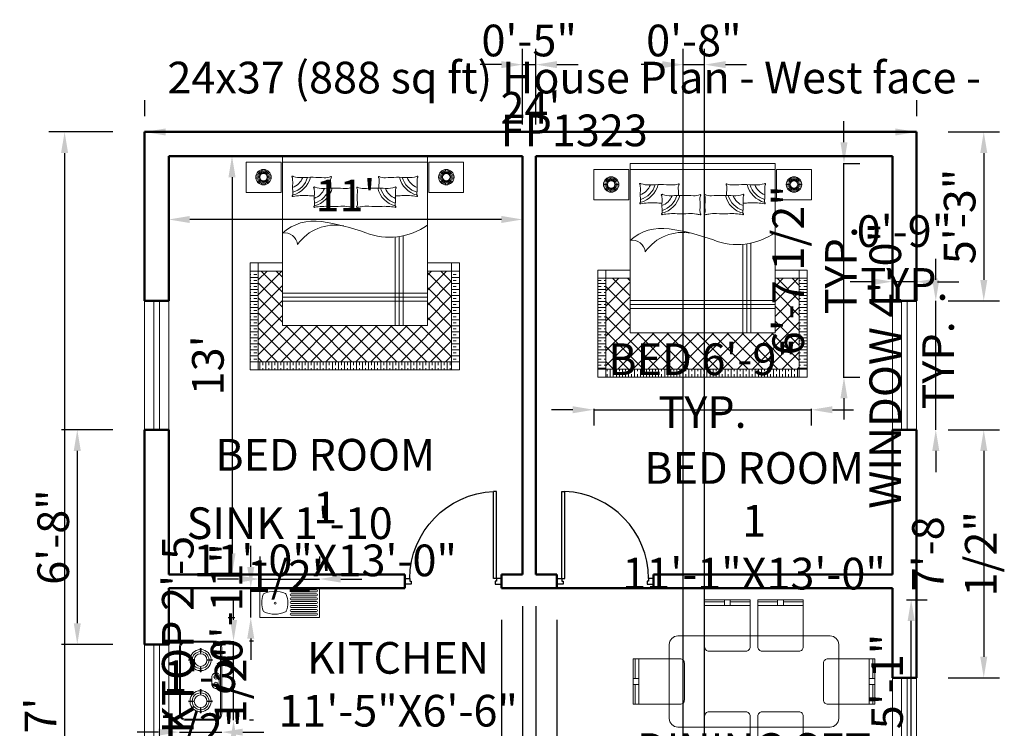
# Model space of a CAD drawing. Units: inches. Extents: x 314 to 688, y 344 to 882.
# Tile 3 of 3: x 321 to 688, y 618 to 882. Entities that reach past the tile are written whole.
import ezdxf

# ---------------------------------------------------------------- set-up
doc = ezdxf.new("R2010")
doc.units = ezdxf.units.IN
doc.header["$MEASUREMENT"] = 0
for name, color, linetype, lineweight in [('A-ANNO-TEXT', 7, 'Continuous', 25), ('A-AREA-IDEN', 7, 'Continuous', 25), ('A-DOOR', 4, 'Continuous', 25), ('A-EQPM', 8, 'Continuous', 18), ('A-FLOR-FIXT', 9, 'Continuous', 18), ('A-FURN', 8, 'Continuous', 18), ('WALL', 7, 'Continuous', 50), ('WINDOW', 2, 'Continuous', 18), ('YQ_DIM', 3, 'Continuous', 18)]:
    doc.layers.add(name, color=color, linetype=linetype, lineweight=lineweight)
doc.styles.add('YQ_DIM', font='SUPEROS.SHX', dxfattribs={"width": 0.8, "bigfont": 'HZDX.SHX'})
doc.dimstyles.new('yqi3_937', dxfattribs={"dimscale": 3.937008, "dimtxt": 3, "dimasz": 2, "dimexe": 1.5, "dimexo": 3, "dimgap": 0.5, "dimtad": 1, "dimdsep": 46, "dimlunit": 4, "dimtxsty": 'YQ_DIM', "dimcen": 0, "dimclrd": 256, "dimclre": 256, "dimclrt": 7, "dimadec": 1, "dimazin": 2, "dimtfac": 1, "dimtix": 1, "dimtmove": 2, "dimatfit": 2, "dimfxl": 1, "dimtolj": 1, "dimtzin": 0, "dimarcsym": 0})

# ---------------------------------------------------------------- blocks, each defined once
blk = doc.blocks.new('*D2')
at = {"layer": 'Defpoints', "color": 0, "transparency": 16777216}
for p in [(367.29, 840.23), (337.46, 396.23), (367.29, 396.23)]:
    blk.add_point(p, dxfattribs=at)
at = {"layer": 'YQ_DIM', "color": 0, "lineweight": -2, "transparency": 16777216}
for p, q in [((355.48, 840.23), (331.55, 840.23)), ((337.46, 832.36), (337.46, 404.11)), ((355.48, 396.23), (331.55, 396.23))]:
    blk.add_line(p, q, dxfattribs=at)
at = {"layer": 'YQ_DIM', "color": 0, "transparency": 16777216}
for points in [[(336.14, 832.36), (338.77, 832.36), (337.46, 840.23)], [(336.14, 404.11), (338.77, 404.11), (337.46, 396.23)]]:
    blk.add_solid(points, dxfattribs=at)
at = {"layer": 'YQ_DIM', "color": 0, "transparency": 16777216, "insert": (328.46, 618.23), "char_height": 11.811, "attachment_point": 5, "rotation": 90, "style": 'YQ_DIM'}
blk.add_mtext("\\A1;37'", dxfattribs=at)
blk = doc.blocks.new('*D3')
at = {"layer": 'Defpoints', "color": 0, "transparency": 16777216}
for p in [(376.29, 831.23), (508.29, 831.23), (376.29, 807.61)]:
    blk.add_point(p, dxfattribs=at)
at = {"layer": 'YQ_DIM', "color": 0, "lineweight": -2, "transparency": 16777216}
for p, q in [((376.29, 819.42), (376.29, 801.71)), ((508.29, 819.42), (508.29, 801.71)), ((500.42, 807.61), (384.17, 807.61))]:
    blk.add_line(p, q, dxfattribs=at)
at = {"layer": 'YQ_DIM', "color": 0, "transparency": 16777216}
for points in [[(384.17, 808.92), (384.17, 806.3), (376.29, 807.61)], [(500.42, 808.92), (500.42, 806.3), (508.29, 807.61)]]:
    blk.add_solid(points, dxfattribs=at)
at = {"layer": 'YQ_DIM', "color": 0, "transparency": 16777216, "insert": (442.29, 816.61), "char_height": 11.811, "attachment_point": 5, "style": 'YQ_DIM'}
blk.add_mtext("\\A1;11'", dxfattribs=at)
blk = doc.blocks.new('*D4')
at = {"layer": 'Defpoints', "color": 0, "transparency": 16777216}
for p in [(376.29, 831.23), (376.29, 675.23), (399.92, 675.23)]:
    blk.add_point(p, dxfattribs=at)
at = {"layer": 'YQ_DIM', "color": 0, "lineweight": -2, "transparency": 16777216}
for p, q in [((388.1, 831.23), (405.82, 831.23)), ((399.92, 823.36), (399.92, 683.11)), ((388.1, 675.23), (405.82, 675.23))]:
    blk.add_line(p, q, dxfattribs=at)
at = {"layer": 'YQ_DIM', "color": 0, "transparency": 16777216}
for points in [[(398.6, 823.36), (401.23, 823.36), (399.92, 831.23)], [(398.6, 683.11), (401.23, 683.11), (399.92, 675.23)]]:
    blk.add_solid(points, dxfattribs=at)
at = {"layer": 'YQ_DIM', "color": 0, "transparency": 16777216, "insert": (390.92, 753.23), "char_height": 11.811, "attachment_point": 5, "rotation": 90, "style": 'YQ_DIM'}
blk.add_mtext("\\A1;13'", dxfattribs=at)
blk = doc.blocks.new('DR_D01')
for p, q in [((-0.45, 0.93), (-0.42, 0.93)), ((-0.45, 0.03), (-0.45, 0.93)), ((-0.42, 0.03), (-0.42, 0.93)), ((-0.5, 0.03), (-0.42, 0.03)), ((-0.5, 0.03), (-0.5, -0.03)), ((-0.45, 0.03), (-0.45, 0)), ((-0.45, 0), (-0.435, 0)), ((-0.435, 0), (-0.435, -0.03)), ((0.435, 0), (0.435, -0.03)), ((0.45, 0), (0.435, 0)), ((0.45, 0.03), (0.45, 0)), ((0.5, 0.03), (0.45, 0.03)), ((0.5, -0.03), (0.5, 0.03)), ((-0.435, -0.03), (-0.5, -0.03)), ((0.435, -0.03), (0.5, -0.03))]:
    blk.add_line(p, q)
blk.add_arc((-0.46, 0.021), 0.91, 0.5915, 87.4664)
blk = doc.blocks.new('WD_WIN4')
for p, q in [((-0.5, 0.5), (0.5, 0.5)), ((-0.5, 0.12), (0.5, 0.12)), ((-0.5, -0.12), (0.5, -0.12)), ((-0.5, -0.5), (0.5, -0.5))]:
    blk.add_line(p, q)
blk = doc.blocks.new('*D8')
at = {"layer": 'Defpoints', "color": 0, "transparency": 16777216}
for p in [(367.29, 840.23), (655.29, 840.23), (655.29, 840.23)]:
    blk.add_point(p, dxfattribs=at)
at = {"layer": 'YQ_DIM', "color": 0, "lineweight": -2, "transparency": 16777216}
for p, q in [((367.29, 852.04), (367.29, 846.14)), ((655.29, 852.04), (655.29, 846.14)), ((375.17, 840.23), (647.42, 840.23))]:
    blk.add_line(p, q, dxfattribs=at)
at = {"layer": 'YQ_DIM', "color": 0, "transparency": 16777216}
for points in [[(375.17, 841.54), (375.17, 838.92), (367.29, 840.23)], [(647.42, 841.54), (647.42, 838.92), (655.29, 840.23)]]:
    blk.add_solid(points, dxfattribs=at)
at = {"layer": 'YQ_DIM', "color": 0, "transparency": 16777216, "insert": (511.29, 849.23), "char_height": 11.811, "attachment_point": 5, "style": 'YQ_DIM'}
blk.add_mtext("\\A1;24'", dxfattribs=at)
blk = doc.blocks.new('BED')
h = blk.add_hatch()
h.set_pattern_fill('TRANS', color=256, scale=12, style=0)
h.set_pattern_definition([(360, (4433.967, -9715.0492), (1e-15, 3), []), (360, (4433.967, -9713.5492), (1e-15, 3), [1.5, -1.5])])
h.paths.add_polyline_path([(48, -103), (52, -103), (52, -58), (48, -58)])
h.paths.add_polyline_path([(-48, -58), (-52, -58), (-52, -103), (-48, -103)])
h = blk.add_hatch()
h.set_pattern_fill('ANSI37', color=256, scale=42, angle=-90, style=0)
h.set_pattern_definition([(315, (7787.1367, 4477.8466), (3.7123106, 3.7123106), []), (45, (7787.1367, 4477.8466), (-3.7123106, 3.7123106), [])])
h.paths.add_polyline_path([(-36, -85), (-36, -58), (-48, -58), (-48, -103), (48, -103), (48, -58), (36, -58), (36, -85)])
h = blk.add_hatch()
h.set_pattern_fill('TRANS', color=256, scale=12, angle=-90, style=0)
h.set_pattern_definition([(270, (4433.967, -9715.0492), (3, -1e-15), []), (270, (4435.467, -9715.0492), (3, -1e-15), [1.5, -1.5])])
h.paths.add_polyline_path([(48, -107), (48, -103), (-48, -103), (-48, -107)])
for p, q in [((-54, -4), (-54, -19)), ((-36.64, -4), (-54, -4)), ((-36.64, -4), (-36.64, -19)), ((-36, -1), (36, -1)), ((-36, -85), (-36, -1)), ((-36, -4), (36, -4)), ((36, -1), (36, -85)), ((36.64, -4), (36.64, -19)), ((36.64, -4), (54, -4)), ((54, -4), (54, -19)), ((-46.88, -10.37), (-48.5, -9.2)), ((-46.62, -10.08), (-47.96, -8.6)), ((-46.31, -9.86), (-47.31, -8.13)), ((-45.96, -9.7), (-46.58, -7.8)), ((-45.58, -9.62), (-45.8, -7.63)), ((-45.2, -9.62), (-45, -7.63)), ((-44.82, -9.7), (-44.21, -7.79)), ((-44.47, -9.85), (-43.48, -8.12)), ((-44.16, -10.08), (-42.83, -8.59)), ((-43.9, -10.36), (-42.29, -9.18)), ((43.9, -10.36), (42.29, -9.18)), ((44.16, -10.08), (42.83, -8.59)), ((44.47, -9.85), (43.48, -8.12)), ((44.82, -9.7), (44.21, -7.79)), ((45.2, -9.62), (45, -7.63)), ((45.58, -9.62), (45.8, -7.63)), ((45.96, -9.7), (46.58, -7.8)), ((46.31, -9.86), (47.31, -8.13)), ((46.62, -10.08), (47.96, -8.6)), ((46.88, -10.37), (48.5, -9.2)), ((-47.23, -11.45), (-49.23, -11.45)), ((-47.19, -11.07), (-49.14, -10.66)), ((-47.19, -11.83), (-49.14, -12.25)), ((-47.07, -10.7), (-48.9, -9.89)), ((-47.07, -12.2), (-48.89, -13.01)), ((-46.87, -12.53), (-48.49, -13.71)), ((-46.62, -12.81), (-47.95, -14.3)), ((-46.3, -13.04), (-47.3, -14.77)), ((-45.95, -13.2), (-46.57, -15.1)), ((-45.58, -13.27), (-45.78, -15.26)), ((-45.19, -13.27), (-44.98, -15.26)), ((-44.82, -13.19), (-44.2, -15.09)), ((-44.47, -13.04), (-43.46, -14.77)), ((-44.16, -12.81), (-42.82, -14.29)), ((-43.9, -12.52), (-42.28, -13.7)), ((-43.71, -10.7), (-41.89, -9.88)), ((-43.71, -12.19), (-41.88, -13)), ((-43.59, -11.06), (-41.64, -10.64)), ((-43.59, -11.83), (-41.63, -12.24)), ((-43.55, -11.44), (-41.55, -11.44)), ((43.55, -11.44), (41.55, -11.44)), ((43.59, -11.83), (41.63, -12.24)), ((43.59, -11.06), (41.64, -10.64)), ((43.71, -12.19), (41.88, -13)), ((43.71, -10.7), (41.89, -9.88)), ((43.9, -12.52), (42.28, -13.7)), ((44.16, -12.81), (42.82, -14.29)), ((44.47, -13.04), (43.46, -14.77)), ((44.82, -13.19), (44.2, -15.09)), ((45.19, -13.27), (44.98, -15.26)), ((45.58, -13.27), (45.78, -15.26)), ((45.95, -13.2), (46.57, -15.1)), ((46.3, -13.04), (47.3, -14.77)), ((46.62, -12.81), (47.95, -14.3)), ((46.87, -12.53), (48.49, -13.71)), ((47.07, -10.7), (48.9, -9.89)), ((47.07, -12.2), (48.89, -13.01)), ((47.19, -11.07), (49.14, -10.66)), ((47.19, -11.83), (49.14, -12.25)), ((47.23, -11.45), (49.23, -11.45)), ((-36.64, -19), (-54, -19)), ((36.64, -19), (54, -19)), ((20, -85), (20, -41.14)), ((22, -85), (22, -40.91)), ((24, -85), (24, -40.55)), ((-52, -54), (-52, -107)), ((-52, -54), (-36, -54)), ((-52, -58), (-36, -58)), ((-48, -54), (-48, -107)), ((36, -54), (52, -54)), ((36, -58), (52, -58)), ((48, -54), (48, -107)), ((52, -54), (52, -107)), ((36, -69), (-36, -69)), ((36, -71), (-36, -71)), ((36, -73), (-36, -73)), ((36, -85), (-36, -85)), ((-52, -103), (52, -103)), ((-52, -107), (52, -107))]:
    blk.add_line(p, q)
for centre, radius in [((-45.39, -11.45), 3.84), ((-45.39, -11.45), 1.84), ((45.39, -11.45), 3.84), ((45.39, -11.45), 1.84)]:
    blk.add_circle(centre, radius)
for centre, radius, start, end in [((-30.92, -11.24), 0.328, 35.8976, 208.6272), ((-42.38, -17.5), 12.73, 27.1629, 28.6272), ((-44.37, -13.89), 13.5, 357.4804, 9.3956), ((10.15, -16.29), 41.07, 177.4804, 184.5075), ((-33.8, -8.61), 8.46, 289.8695, 338.9843), ((-33.8, -8.61), 12.06, 283.8498, 346.0842), ((-33.8, -8.61), 10.71, 286.0319, 344.1205), ((-26.84, 0.13), 11.82, 251.1782, 273.3982), ((-20.92, -99.64), 88.13, 86.2964, 93.3982), ((-14.79, -4.98), 6.73, 266.2964, 294.303), ((-8.24, -13.16), 3.86, 159.0146, 186.273), ((-36.64, -16.28), 24.71, 358.5721, 6.273), ((-11.92, -11.33), 0.242, 335.7259, 114.303), ((-5.69, -14.14), 6.59, 155.7259, 159.0146), ((11.92, -11.33), 0.242, 65.697, 204.2741), ((5.69, -14.14), 6.59, 20.9854, 24.2741), ((8.24, -13.16), 3.86, 353.727, 20.9854), ((36.64, -16.28), 24.71, 173.727, 181.4279), ((14.79, -4.98), 6.73, 245.697, 273.7036), ((20.92, -99.64), 88.13, 86.6018, 93.7036), ((33.8, -8.61), 12.06, 193.9158, 256.1502), ((33.8, -8.61), 10.71, 195.8795, 253.9681), ((33.8, -8.61), 8.46, 201.0157, 250.1305), ((26.84, 0.13), 11.82, 266.6018, 288.8218), ((30.92, -11.24), 0.328, 331.3728, 144.1024), ((-10.15, -16.29), 41.07, 355.4925, 2.5196), ((44.37, -13.89), 13.5, 170.6044, 182.5196), ((42.38, -17.5), 12.73, 151.3728, 152.8371), ((-32.67, -19.67), 1.88, 339.2246, 4.5075), ((-20.16, -16.62), 0.328, 35.8976, 208.6272), ((-31.62, -22.87), 12.73, 27.1629, 28.6272), ((-33.61, -19.26), 13.5, 357.4804, 9.3956), ((-23.04, -13.99), 8.46, 289.8695, 338.9843), ((-23.04, -13.99), 12.06, 283.8498, 346.0842), ((-23.04, -13.99), 10.71, 286.0319, 344.1205), ((-16.08, -5.24), 11.82, 251.1782, 273.3982), ((-10.15, -105.01), 88.13, 86.2964, 93.3982), ((-4.03, -10.35), 6.73, 266.2964, 294.303), ((2.52, -18.53), 3.86, 159.0146, 186.273), ((-25.88, -21.66), 24.71, 354.3784, 6.273), ((-1.16, -16.7), 0.242, 335.7259, 114.303), ((5.07, -19.51), 6.59, 155.7259, 159.0146), ((1.16, -16.7), 0.242, 65.697, 204.2741), ((-5.07, -19.51), 6.59, 20.9854, 24.2741), ((-2.52, -18.53), 3.86, 353.727, 20.9854), ((25.88, -21.66), 24.71, 173.727, 185.6216), ((4.03, -10.35), 6.73, 245.697, 273.7036), ((10.15, -105.01), 88.13, 86.6018, 93.7036), ((23.04, -13.99), 12.06, 193.9158, 256.1502), ((23.04, -13.99), 10.71, 195.8795, 253.9681), ((23.04, -13.99), 8.46, 201.0157, 250.1305), ((16.08, -5.24), 11.82, 266.6018, 288.8218), ((20.16, -16.62), 0.328, 331.3728, 144.1024), ((33.61, -19.26), 13.5, 170.6044, 182.5196), ((31.62, -22.87), 12.73, 151.3728, 152.8371), ((32.67, -19.67), 1.88, 175.4925, 200.7754), ((-30.88, -20.82), 0.25, 147.6219, 311.9343), ((-32.72, -19.65), 1.93, 327.6219, 339.2246), ((-25.16, -53.53), 33, 93.5164, 99.6766), ((-25.27, -51.86), 31.33, 86.4836, 93.5164), ((-21.12, 15.68), 36.34, 266.4836, 271.5234), ((20.91, -21.66), 41.07, 177.4804, 184.5075), ((2.55, -24.46), 3.86, 174.3784, 204.7617), ((-2.55, -24.46), 3.86, 335.2383, 5.6216), ((-20.91, -21.66), 41.07, 355.4925, 2.5196), ((21.12, 15.68), 36.34, 268.4766, 273.5164), ((25.27, -51.86), 31.33, 86.4836, 93.5164), ((25.16, -53.53), 33, 80.3234, 86.4836), ((30.88, -20.82), 0.25, 228.0657, 32.3781), ((32.72, -19.65), 1.93, 200.7754, 212.3781), ((-20.12, -26.19), 0.25, 147.6219, 311.9343), ((-21.96, -25.02), 1.93, 327.6219, 339.2246), ((-21.91, -25.04), 1.88, 339.2246, 4.5075), ((-14.4, -58.9), 33, 93.5164, 99.6766), ((-14.51, -57.23), 31.33, 86.4836, 93.5164), ((-10.35, 10.3), 36.34, 266.4836, 275.306), ((-5.78, -38.98), 13.15, 77.9645, 95.306), ((2.5, -0.17), 26.53, 257.9645, 261.9243), ((-1.09, -26.25), 0.228, 231.9005, 52.8902), ((1.09, -26.25), 0.228, 127.1098, 308.0995), ((-2.5, -0.17), 26.53, 278.0757, 282.0355), ((5.78, -38.98), 13.15, 84.694, 102.0355), ((10.35, 10.3), 36.34, 264.694, 273.5164), ((14.51, -57.23), 31.33, 86.4836, 93.5164), ((14.4, -58.9), 33, 80.3234, 86.4836), ((20.12, -26.19), 0.25, 228.0657, 32.3781), ((21.91, -25.04), 1.88, 175.4925, 200.7754), ((21.96, -25.02), 1.93, 200.7754, 212.3781), ((-20.27, -56.85), 23.66, 81.0857, 131.6581), ((-32.56, -143.87), 111.55, 70.0977, 81.7735), ((-34.97, -45.63), 6.55, 6.3172, 99.0807), ((-9.91, -57.83), 22.61, 78.6456, 145.1521), ((17.27, -9.21), 32.05, 248.2778, 305.7663)]:
    blk.add_arc(centre, radius, start, end)
blk = doc.blocks.new('yq_cooker_01')
for p, q in [((426.3, 34.3), (465.5, 34.3)), ((426.3, -34.3), (465.5, -34.3))]:
    blk.add_line(p, q)
for points in [[(440, -375), (160, -375, -0.414214), (100, -315), (100, 315, -0.414214), (160, 375), (440, 375, -0.414214), (500, 315), (500, -315, -0.414214)], [(440, -365), (160, -365, -0.414214), (110, -315), (110, 315, -0.414214), (160, 365), (440, 365, -0.414214), (490, 315), (490, -315, -0.414214)]]:
    blk.add_lwpolyline(points, format="xyb", close=True)
for points in [[(300.8, 261.3), (305.4, 305), (294.6, 305), (299.2, 261.3)], [(233.7, 195.8), (190, 200.4), (190, 189.6), (233.7, 194.2)], [(366.3, 194.2), (410, 189.6), (410, 200.4), (366.3, 195.8)], [(299.2, 128.7), (294.6, 85), (305.4, 85), (300.8, 128.7)], [(299.2, -128.7), (294.6, -85), (305.4, -85), (300.8, -128.7)], [(233.7, -195.8), (190, -200.4), (190, -189.6), (233.7, -194.2)], [(300.8, -261.3), (305.4, -305), (294.6, -305), (299.2, -261.3)], [(366.3, -194.2), (410, -189.6), (410, -200.4), (366.3, -195.8)]]:
    blk.add_lwpolyline(points, close=True)
blk.add_lwpolyline([(406.7, -34.3, 0.414214), (445.9, -73.5), (455.5, -73.5, 0.414214), (475.1, -53.9), (475.1, 53.9, 0.414214), (455.5, 73.5), (445.9, 73.5, 0.414214), (406.7, 34.3), (406.7, -34.3)], format="xyb")
for centre, radius in [((300, 195), 60), ((445.9, 34.3), 19.6), ((445.9, -34.3), 19.6), ((300, -195), 60)]:
    blk.add_circle(centre, radius)
for centre, radius, start, end in [((300, 195), 100, 92.4978, 177.5022), ((300, 195), 100, 2.4978, 87.5022), ((300, 195), 100, 182.4978, 267.5022), ((300, 195), 80, 91.59131, 178.40869), ((300, 195), 80, 181.59131, 268.40869), ((300, 195), 80, 1.59131, 88.40869), ((300, 195), 80, 271.59131, 358.40869), ((300, 195), 100, 272.4978, 357.5022), ((300, -195), 100, 92.4978, 177.5022), ((300, -195), 80, 91.59131, 178.40869), ((300, -195), 80, 1.59131, 88.40869), ((300, -195), 100, 2.4978, 87.5022), ((300, -195), 100, 182.4978, 267.5022), ((300, -195), 80, 181.59131, 268.40869), ((300, -195), 80, 271.59131, 358.40869), ((300, -195), 100, 272.4978, 357.5022)]:
    blk.add_arc(centre, radius, start, end)
blk = doc.blocks.new('sink7a')
for p, q in [((12297, -765), (22250, -765)), ((12297, -1527), (22250, -1527)), ((12297, -2289), (22250, -2289)), ((12297, -3051), (22250, -3051)), ((12297, -3813), (22250, -3813)), ((12297, -4575), (22250, -4575)), ((12297, -5337), (22250, -5337)), ((12297, -6099), (22250, -6099)), ((12297, -6861), (22250, -6861)), ((12297, -7623), (22250, -7623)), ((12297, -8385), (22250, -8385)), ((12297, -9147), (22250, -9147)), ((12297, -9909), (22250, -9909)), ((12297, -10671), (22250, -10671))]:
    blk.add_line(p, q)
blk.add_lwpolyline([(0, 0), (0, -11557), (23495, -11557), (23495, 0)], close=True)
blk.add_lwpolyline([(1692, -9356, -0.193356), (1368, -9011, -0.1886606), (1376, -2541, -0.1929606), (1700, -2197, -0.2205414), (10111, -2197, -0.1929606), (10435, -2541, -0.1886606), (10443, -9011, -0.193356), (10119, -9356, -0.2209789)], format="xyb", close=True)
blk.add_circle((6064, -5888), 381)
for centre, start, end in [((12297, -1146), 90, 270), ((12297, -2670), 90, 270), ((12297, -4194), 90, 270), ((22250, -1146), 270, 90), ((22250, -2670), 270, 90), ((22250, -4194), 270, 90), ((12297, -5718), 90, 270), ((12297, -7242), 90, 270), ((22250, -5718), 270, 90), ((22250, -7242), 270, 90), ((12297, -8766), 90, 270), ((12297, -10290), 90, 270), ((22250, -8766), 270, 90), ((22250, -10290), 270, 90)]:
    blk.add_arc(centre, 381, start, end)
blk = doc.blocks.new('East 1200 Sq.ft$0$din1')
for p, q in [((-487.5, 578.6), (-487.5, 807.1)), ((-487.5, 807.1), (-291.1, 807.1)), ((-487.5, 785.7), (-291.1, 785.7)), ((-291.1, 750), (-291.1, 807.1)), ((-291.1, 807.1), (-233.9, 807.1)), ((-233.9, 750), (-233.9, 807.1)), ((-233.9, 807.1), (-37.5, 807.1)), ((-233.9, 785.7), (-37.5, 785.7)), ((-37.5, 807.1), (-37.5, 578.6)), ((37.5, 807.1), (37.5, 578.6)), ((233.9, 807.1), (37.5, 807.1)), ((233.9, 785.7), (37.5, 785.7)), ((233.9, 750), (233.9, 807.1)), ((291.1, 807.1), (233.9, 807.1)), ((487.5, 807.1), (291.1, 807.1)), ((291.1, 750), (291.1, 807.1)), ((487.5, 785.7), (291.1, 785.7)), ((487.5, 578.6), (487.5, 807.1)), ((-487.5, 750), (-37.5, 750)), ((487.5, 750), (37.5, 750)), ((-966.1, 225), (-1194.6, 225)), ((-1194.6, 225), (-1194.6, 28.6)), ((-1173.2, 225), (-1173.2, 28.6)), ((-1137.5, 225), (-1137.5, -225)), ((966.1, 225), (1194.6, 225)), ((1137.5, 225), (1137.5, -225)), ((1173.2, 225), (1173.2, 28.6)), ((1194.6, 225), (1194.6, 28.6)), ((-1137.5, 28.6), (-1194.6, 28.6)), ((-1194.6, 28.6), (-1194.6, -28.6)), ((1137.5, 28.6), (1194.6, 28.6)), ((1194.6, 28.6), (1194.6, -28.6)), ((-1137.5, -28.6), (-1194.6, -28.6)), ((-1194.6, -28.6), (-1194.6, -225)), ((-1173.2, -28.6), (-1173.2, -225)), ((1137.5, -28.6), (1194.6, -28.6)), ((1173.2, -28.6), (1173.2, -225)), ((1194.6, -28.6), (1194.6, -225)), ((-1194.6, -225), (-966.1, -225)), ((1194.6, -225), (966.1, -225)), ((-487.5, -578.6), (-487.5, -807.1)), ((-37.5, -807.1), (-37.5, -578.6)), ((37.5, -807.1), (37.5, -578.6)), ((487.5, -578.6), (487.5, -807.1)), ((-487.5, -750), (-37.5, -750)), ((-291.1, -750), (-291.1, -807.1)), ((-233.9, -750), (-233.9, -807.1)), ((487.5, -750), (37.5, -750)), ((233.9, -750), (233.9, -807.1)), ((291.1, -750), (291.1, -807.1)), ((-487.5, -785.7), (-291.1, -785.7)), ((-487.5, -807.1), (-291.1, -807.1)), ((-291.1, -807.1), (-233.9, -807.1)), ((-233.9, -785.7), (-37.5, -785.7)), ((-233.9, -807.1), (-37.5, -807.1)), ((233.9, -785.7), (37.5, -785.7)), ((233.9, -807.1), (37.5, -807.1)), ((291.1, -807.1), (233.9, -807.1)), ((487.5, -785.7), (291.1, -785.7)), ((487.5, -807.1), (291.1, -807.1))]:
    blk.add_line(p, q)
for points in [[(-37.5, 578.6), (-37.5, 342.9, -0.414214), (-80.4, 300), (-444.6, 300, -0.414214), (-487.5, 342.9), (-487.5, 578.6)], [(37.5, 578.6), (37.5, 342.9, 0.414214), (80.4, 300), (444.6, 300, 0.414214), (487.5, 342.9), (487.5, 578.6)], [(-966.1, -225), (-730.4, -225, 0.414214), (-687.5, -182.1), (-687.5, 182.1, 0.414214), (-730.4, 225), (-966.1, 225)], [(966.1, -225), (730.4, -225, -0.414214), (687.5, -182.1), (687.5, 182.1, -0.414214), (730.4, 225), (966.1, 225)], [(-37.5, -578.6), (-37.5, -342.9, 0.414214), (-80.4, -300), (-444.6, -300, 0.414214), (-487.5, -342.9), (-487.5, -578.6)], [(37.5, -578.6), (37.5, -342.9, -0.414214), (80.4, -300), (444.6, -300, -0.414214), (487.5, -342.9), (487.5, -578.6)]]:
    blk.add_lwpolyline(points, format="xyb")
blk.add_lwpolyline([(751.8, -450), (-751.8, -450, -0.414214), (-837.5, -364.3), (-837.5, 364.3, -0.414214), (-751.8, 450), (751.8, 450, -0.414214), (837.5, 364.3), (837.5, -364.3, -0.414214)], format="xyb", close=True)
blk = doc.blocks.new('*D16')
at = {"layer": 'Defpoints', "color": 0, "transparency": 16777216}
for p in [(655.29, 777.23), (662.49, 777.23), (655.29, 729.23)]:
    blk.add_point(p, dxfattribs=at)
at = {"layer": 'YQ_DIM', "lineweight": -2, "transparency": 16777216}
for p, q in [((662.49, 785.11), (662.49, 792.98)), ((662.49, 729.23), (662.49, 777.23)), ((667.1, 777.23), (668.4, 777.23)), ((667.1, 729.23), (668.4, 729.23)), ((662.49, 721.36), (662.49, 713.48))]:
    blk.add_line(p, q, dxfattribs=at)
at = {"layer": 'YQ_DIM', "transparency": 16777216}
for points in [[(661.18, 785.11), (663.81, 785.11), (662.49, 777.23)], [(661.18, 721.36), (663.81, 721.36), (662.49, 729.23)]]:
    blk.add_solid(points, dxfattribs=at)
at = {"layer": 'YQ_DIM', "color": 7, "transparency": 16777216, "insert": (653.5, 753.23), "char_height": 11.811, "attachment_point": 5, "rotation": 90, "style": 'YQ_DIM'}
blk.add_mtext('\\A1;WINDOW 4\'-0" TYP.', dxfattribs=at)
blk = doc.blocks.new('*D17')
at = {"layer": 'Defpoints', "color": 0, "transparency": 16777216}
for p in [(646.29, 784.43), (646.29, 777.23), (655.29, 777.23)]:
    blk.add_point(p, dxfattribs=at)
at = {"layer": 'YQ_DIM', "lineweight": -2, "transparency": 16777216}
for p, q in [((646.29, 789.04), (646.29, 790.34)), ((655.29, 789.04), (655.29, 790.34)), ((638.42, 784.43), (630.55, 784.43)), ((655.29, 784.43), (646.29, 784.43)), ((663.17, 784.43), (671.04, 784.43))]:
    blk.add_line(p, q, dxfattribs=at)
at = {"layer": 'YQ_DIM', "transparency": 16777216}
for points in [[(638.42, 785.74), (638.42, 783.12), (646.29, 784.43)], [(663.17, 785.74), (663.17, 783.12), (655.29, 784.43)]]:
    blk.add_solid(points, dxfattribs=at)
at = {"layer": 'YQ_DIM', "color": 7, "transparency": 16777216, "insert": (650.79, 793.43), "char_height": 11.811, "attachment_point": 5, "style": 'YQ_DIM'}
blk.add_mtext('\\A1;0\'-9" TYP.', dxfattribs=at)
blk = doc.blocks.new('*D26')
at = {"layer": 'Defpoints', "color": 0, "transparency": 16777216}
for p in [(534.9, 748.86), (616.06, 748.86), (616.06, 736.68)]:
    blk.add_point(p, dxfattribs=at)
at = {"layer": 'YQ_DIM', "lineweight": -2, "transparency": 16777216}
for p, q in [((527.03, 736.68), (519.15, 736.68)), ((534.9, 737.04), (534.9, 730.78)), ((534.9, 736.68), (616.06, 736.68)), ((616.06, 737.04), (616.06, 730.78)), ((623.94, 736.68), (631.81, 736.68))]:
    blk.add_line(p, q, dxfattribs=at)
at = {"layer": 'YQ_DIM', "transparency": 16777216}
for points in [[(527.03, 737.99), (527.03, 735.37), (534.9, 736.68)], [(623.94, 737.99), (623.94, 735.37), (616.06, 736.68)]]:
    blk.add_solid(points, dxfattribs=at)
at = {"layer": 'YQ_DIM', "color": 7, "transparency": 16777216, "insert": (575.48, 745.68), "char_height": 11.811, "attachment_point": 5, "style": 'YQ_DIM'}
blk.add_mtext('\\A1;BED 6\'-9" TYP.', dxfattribs=at)
blk = doc.blocks.new('*D27')
at = {"layer": 'Defpoints', "color": 0, "transparency": 16777216}
for p in [(616.06, 828.51), (628.24, 828.51), (616.06, 748.86)]:
    blk.add_point(p, dxfattribs=at)
at = {"layer": 'YQ_DIM', "lineweight": -2, "transparency": 16777216}
for p, q in [((628.24, 836.39), (628.24, 844.26)), ((627.88, 828.51), (634.14, 828.51)), ((628.24, 748.86), (628.24, 828.51)), ((627.88, 748.86), (634.14, 748.86)), ((628.24, 740.98), (628.24, 733.11))]:
    blk.add_line(p, q, dxfattribs=at)
at = {"layer": 'YQ_DIM', "transparency": 16777216}
for points in [[(626.93, 836.39), (629.55, 836.39), (628.24, 828.51)], [(626.93, 740.98), (629.55, 740.98), (628.24, 748.86)]]:
    blk.add_solid(points, dxfattribs=at)
at = {"layer": 'YQ_DIM', "color": 7, "transparency": 16777216, "insert": (617.27, 788.68), "char_height": 11.811, "attachment_point": 5, "rotation": 90, "style": 'YQ_DIM'}
blk.add_mtext('\\A1;6\'-7 1/2" TYP.', dxfattribs=at)
blk = doc.blocks.new('*D30')
at = {"layer": 'Defpoints', "color": 0, "transparency": 16777216}
for p in [(396.07, 650.46), (400.5, 650.46), (396.07, 620.93)]:
    blk.add_point(p, dxfattribs=at)
at = {"layer": 'YQ_DIM', "lineweight": -2, "transparency": 16777216}
for p, q in [((400.5, 658.33), (400.5, 666.2)), ((400.5, 620.93), (400.5, 650.46)), ((407.88, 650.46), (406.41, 650.46)), ((407.88, 620.93), (406.41, 620.93)), ((400.5, 613.05), (400.5, 605.18))]:
    blk.add_line(p, q, dxfattribs=at)
at = {"layer": 'YQ_DIM', "transparency": 16777216}
for points in [[(399.19, 658.33), (401.81, 658.33), (400.5, 650.46)], [(399.19, 613.05), (401.81, 613.05), (400.5, 620.93)]]:
    blk.add_solid(points, dxfattribs=at)
at = {"layer": 'YQ_DIM', "color": 7, "transparency": 16777216, "insert": (389.53, 635.69), "char_height": 11.811, "attachment_point": 5, "rotation": 90, "style": 'YQ_DIM'}
blk.add_mtext('\\A1;COOKTOP 2\'-5 1/2"', dxfattribs=at)
blk = doc.blocks.new('*D31')
at = {"layer": 'Defpoints', "color": 0, "transparency": 16777216}
for p in [(380.33, 620.93), (396.07, 620.93), (396.07, 616.5)]:
    blk.add_point(p, dxfattribs=at)
at = {"layer": 'YQ_DIM', "lineweight": -2, "transparency": 16777216}
for p, q in [((372.45, 616.5), (364.58, 616.5)), ((380.33, 616.5), (396.07, 616.5)), ((403.95, 616.5), (411.82, 616.5)), ((380.33, 609.12), (380.33, 610.59)), ((396.07, 609.12), (396.07, 610.59))]:
    blk.add_line(p, q, dxfattribs=at)
at = {"layer": 'YQ_DIM', "transparency": 16777216}
for points in [[(372.45, 617.81), (372.45, 615.19), (380.33, 616.5)], [(403.95, 617.81), (403.95, 615.19), (396.07, 616.5)]]:
    blk.add_solid(points, dxfattribs=at)
at = {"layer": 'YQ_DIM', "color": 7, "transparency": 16777216, "insert": (388.2, 627.47), "char_height": 11.811, "attachment_point": 5, "style": 'YQ_DIM'}
blk.add_mtext('\\A1;1\'-3 1/2"', dxfattribs=at)
blk = doc.blocks.new('*D32')
at = {"layer": 'Defpoints', "color": 0, "transparency": 16777216}
for p in [(432.59, 673.58), (410.26, 670.23), (432.59, 670.23)]:
    blk.add_point(p, dxfattribs=at)
at = {"layer": 'YQ_DIM', "lineweight": -2, "transparency": 16777216}
for p, q in [((410.26, 682.04), (410.26, 679.49)), ((432.59, 682.04), (432.59, 679.49)), ((402.39, 673.58), (394.52, 673.58)), ((410.26, 673.58), (432.59, 673.58)), ((440.46, 673.58), (448.34, 673.58))]:
    blk.add_line(p, q, dxfattribs=at)
at = {"layer": 'YQ_DIM', "transparency": 16777216}
for points in [[(402.39, 674.89), (402.39, 672.27), (410.26, 673.58)], [(440.46, 674.89), (440.46, 672.27), (432.59, 673.58)]]:
    blk.add_solid(points, dxfattribs=at)
at = {"layer": 'YQ_DIM', "color": 7, "transparency": 16777216, "insert": (421.43, 684.55), "char_height": 11.811, "attachment_point": 5, "style": 'YQ_DIM'}
blk.add_mtext('\\A1;SINK 1\'-10 1/2"', dxfattribs=at)
blk = doc.blocks.new('*D33')
at = {"layer": 'Defpoints', "color": 0, "transparency": 16777216}
for p in [(406.92, 670.23), (410.26, 670.23), (410.26, 659.25)]:
    blk.add_point(p, dxfattribs=at)
at = {"layer": 'YQ_DIM', "lineweight": -2, "transparency": 16777216}
for p, q in [((406.92, 678.11), (406.92, 685.98)), ((398.45, 670.23), (401.01, 670.23)), ((406.92, 659.25), (406.92, 670.23)), ((398.45, 659.25), (401.01, 659.25)), ((406.92, 651.38), (406.92, 643.5))]:
    blk.add_line(p, q, dxfattribs=at)
at = {"layer": 'YQ_DIM', "transparency": 16777216}
for points in [[(405.6, 678.11), (408.23, 678.11), (406.92, 670.23)], [(405.6, 651.38), (408.23, 651.38), (406.92, 659.25)]]:
    blk.add_solid(points, dxfattribs=at)
at = {"layer": 'YQ_DIM', "color": 7, "transparency": 16777216, "insert": (397.92, 664.74), "char_height": 11.811, "attachment_point": 5, "rotation": 90, "style": 'YQ_DIM'}
blk.add_mtext('\\A1;0\'-11"', dxfattribs=at)
blk = doc.blocks.new('*D34')
at = {"layer": 'Defpoints', "color": 0, "transparency": 16777216}
for p in [(549.56, 604.9), (639.78, 604.9), (639.78, 591.37)]:
    blk.add_point(p, dxfattribs=at)
at = {"layer": 'YQ_DIM', "lineweight": -2, "transparency": 16777216}
for p, q in [((549.56, 593.09), (549.56, 585.46)), ((639.78, 593.09), (639.78, 585.46)), ((541.68, 591.37), (533.81, 591.37)), ((549.56, 591.37), (639.78, 591.37)), ((647.65, 591.37), (655.53, 591.37))]:
    blk.add_line(p, q, dxfattribs=at)
at = {"layer": 'YQ_DIM', "transparency": 16777216}
for points in [[(541.68, 592.68), (541.68, 590.05), (549.56, 591.37)], [(647.65, 592.68), (647.65, 590.05), (639.78, 591.37)]]:
    blk.add_solid(points, dxfattribs=at)
at = {"layer": 'YQ_DIM', "color": 7, "transparency": 16777216, "insert": (594.67, 600.37), "char_height": 11.811, "attachment_point": 5, "style": 'YQ_DIM'}
blk.add_mtext('\\A1;DINING SET 7\'-6"', dxfattribs=at)
blk = doc.blocks.new('*D35')
at = {"layer": 'Defpoints', "color": 0, "transparency": 16777216}
for p in [(639.78, 665.86), (653.31, 665.86), (639.78, 604.9)]:
    blk.add_point(p, dxfattribs=at)
at = {"layer": 'YQ_DIM', "lineweight": -2, "transparency": 16777216}
for p, q in [((651.59, 665.86), (659.22, 665.86)), ((653.31, 612.77), (653.31, 657.98)), ((651.59, 604.9), (659.22, 604.9))]:
    blk.add_line(p, q, dxfattribs=at)
at = {"layer": 'YQ_DIM', "transparency": 16777216}
for points in [[(652, 657.98), (654.62, 657.98), (653.31, 665.86)], [(652, 612.77), (654.62, 612.77), (653.31, 604.9)]]:
    blk.add_solid(points, dxfattribs=at)
at = {"layer": 'YQ_DIM', "color": 7, "transparency": 16777216, "insert": (644.31, 635.38), "char_height": 11.811, "attachment_point": 5, "rotation": 90, "style": 'YQ_DIM'}
blk.add_mtext('\\A1;5\'-1"', dxfattribs=at)
blk = doc.blocks.new('*D36')
at = {"layer": 'Defpoints', "color": 0, "transparency": 16777216}
for p in [(655.29, 840.23), (655.29, 777.23), (680.39, 777.23)]:
    blk.add_point(p, dxfattribs=at)
at = {"layer": 'YQ_DIM', "lineweight": -2, "transparency": 16777216}
for p, q in [((667.1, 840.23), (686.3, 840.23)), ((680.39, 832.36), (680.39, 785.11)), ((667.1, 777.23), (686.3, 777.23))]:
    blk.add_line(p, q, dxfattribs=at)
at = {"layer": 'YQ_DIM', "transparency": 16777216}
for points in [[(679.08, 832.36), (681.71, 832.36), (680.39, 840.23)], [(679.08, 785.11), (681.71, 785.11), (680.39, 777.23)]]:
    blk.add_solid(points, dxfattribs=at)
at = {"layer": 'YQ_DIM', "color": 7, "transparency": 16777216, "insert": (671.4, 808.73), "char_height": 11.811, "attachment_point": 5, "rotation": 90, "style": 'YQ_DIM'}
blk.add_mtext('\\A1;5\'-3"', dxfattribs=at)
blk = doc.blocks.new('*D37')
at = {"layer": 'Defpoints', "color": 0, "transparency": 16777216}
for p in [(655.29, 729.23), (655.29, 636.73), (680.39, 636.73)]:
    blk.add_point(p, dxfattribs=at)
at = {"layer": 'YQ_DIM', "lineweight": -2, "transparency": 16777216}
for p, q in [((667.1, 729.23), (686.3, 729.23)), ((680.39, 721.36), (680.39, 644.61)), ((667.1, 636.73), (686.3, 636.73))]:
    blk.add_line(p, q, dxfattribs=at)
at = {"layer": 'YQ_DIM', "transparency": 16777216}
for points in [[(679.08, 721.36), (681.71, 721.36), (680.39, 729.23)], [(679.08, 644.61), (681.71, 644.61), (680.39, 636.73)]]:
    blk.add_solid(points, dxfattribs=at)
at = {"layer": 'YQ_DIM', "color": 7, "transparency": 16777216, "insert": (669.43, 682.98), "char_height": 11.811, "attachment_point": 5, "rotation": 90, "style": 'YQ_DIM'}
blk.add_mtext('\\A1;7\'-8 1/2"', dxfattribs=at)
blk = doc.blocks.new('*D41')
at = {"layer": 'Defpoints', "color": 0, "transparency": 16777216}
for p in [(513.29, 865.33), (508.29, 831.23), (513.29, 831.23)]:
    blk.add_point(p, dxfattribs=at)
at = {"layer": 'YQ_DIM', "lineweight": -2, "transparency": 16777216}
for p, q in [((508.29, 843.04), (508.29, 871.24)), ((513.29, 843.04), (513.29, 871.24)), ((500.42, 865.33), (492.55, 865.33)), ((508.29, 865.33), (513.29, 865.33)), ((521.17, 865.33), (529.04, 865.33))]:
    blk.add_line(p, q, dxfattribs=at)
at = {"layer": 'YQ_DIM', "transparency": 16777216}
for points in [[(500.42, 866.64), (500.42, 864.02), (508.29, 865.33)], [(521.17, 866.64), (521.17, 864.02), (513.29, 865.33)]]:
    blk.add_solid(points, dxfattribs=at)
at = {"layer": 'YQ_DIM', "color": 7, "transparency": 16777216, "insert": (510.79, 874.33), "char_height": 11.811, "attachment_point": 5, "style": 'YQ_DIM'}
blk.add_mtext('\\A1;0\'-5"', dxfattribs=at)
blk = doc.blocks.new('*D42')
at = {"layer": 'Defpoints', "color": 0, "transparency": 16777216}
for p in [(367.29, 729.23), (342.19, 649.23), (367.29, 649.23)]:
    blk.add_point(p, dxfattribs=at)
at = {"layer": 'YQ_DIM', "lineweight": -2, "transparency": 16777216}
for p, q in [((355.48, 729.23), (336.29, 729.23)), ((342.19, 721.36), (342.19, 657.11)), ((355.48, 649.23), (336.29, 649.23))]:
    blk.add_line(p, q, dxfattribs=at)
at = {"layer": 'YQ_DIM', "transparency": 16777216}
for points in [[(340.88, 721.36), (343.51, 721.36), (342.19, 729.23)], [(340.88, 657.11), (343.51, 657.11), (342.19, 649.23)]]:
    blk.add_solid(points, dxfattribs=at)
at = {"layer": 'YQ_DIM', "color": 7, "transparency": 16777216, "insert": (333.2, 689.23), "char_height": 11.811, "attachment_point": 5, "rotation": 90, "style": 'YQ_DIM'}
blk.add_mtext('\\A1;6\'-8"', dxfattribs=at)
blk = doc.blocks.new('*D49')
at = {"layer": 'Defpoints', "color": 0, "transparency": 16777216}
for p in [(508.29, 675.23), (500.42, 670.23), (508.29, 371.13)]:
    blk.add_point(p, dxfattribs=at)
at = {"layer": 'YQ_DIM', "lineweight": -2, "transparency": 16777216}
for p, q in [((508.29, 663.42), (508.29, 365.23)), ((500.42, 658.42), (500.42, 365.23)), ((492.55, 371.13), (484.67, 371.13)), ((500.42, 371.13), (508.29, 371.13)), ((516.17, 371.13), (524.04, 371.13))]:
    blk.add_line(p, q, dxfattribs=at)
at = {"layer": 'YQ_DIM', "transparency": 16777216}
for points in [[(492.55, 372.44), (492.55, 369.82), (500.42, 371.13)], [(516.17, 372.44), (516.17, 369.82), (508.29, 371.13)]]:
    blk.add_solid(points, dxfattribs=at)
at = {"layer": 'YQ_DIM', "color": 7, "transparency": 16777216, "insert": (504.36, 380.13), "char_height": 11.811, "attachment_point": 5, "style": 'YQ_DIM'}
blk.add_mtext('\\A1;0\'-8"', dxfattribs=at)
blk = doc.blocks.new('*D50')
at = {"layer": 'Defpoints', "color": 0, "transparency": 16777216}
for p in [(513.29, 675.23), (521.17, 670.23), (521.17, 371.13)]:
    blk.add_point(p, dxfattribs=at)
at = {"layer": 'YQ_DIM', "lineweight": -2, "transparency": 16777216}
for p, q in [((513.29, 663.42), (513.29, 365.23)), ((521.17, 658.42), (521.17, 365.23)), ((505.42, 371.13), (497.55, 371.13)), ((513.29, 371.13), (521.17, 371.13)), ((529.04, 371.13), (536.92, 371.13))]:
    blk.add_line(p, q, dxfattribs=at)
at = {"layer": 'YQ_DIM', "transparency": 16777216}
for points in [[(505.42, 372.44), (505.42, 369.82), (513.29, 371.13)], [(529.04, 372.44), (529.04, 369.82), (521.17, 371.13)]]:
    blk.add_solid(points, dxfattribs=at)
at = {"layer": 'YQ_DIM', "color": 7, "transparency": 16777216, "insert": (517.23, 380.13), "char_height": 11.811, "attachment_point": 5, "style": 'YQ_DIM'}
blk.add_mtext('\\A1;0\'-8"', dxfattribs=at)
blk = doc.blocks.new('*D52')
at = {"layer": 'Defpoints', "color": 0, "transparency": 16777216}
for p in [(576.17, 865.33), (568.29, 455.23), (576.17, 455.23)]:
    blk.add_point(p, dxfattribs=at)
at = {"layer": 'YQ_DIM', "lineweight": -2, "transparency": 16777216}
for p, q in [((568.29, 467.04), (568.29, 871.24)), ((576.17, 467.04), (576.17, 871.24)), ((560.42, 865.33), (552.55, 865.33)), ((568.29, 865.33), (576.17, 865.33)), ((584.04, 865.33), (591.92, 865.33))]:
    blk.add_line(p, q, dxfattribs=at)
at = {"layer": 'YQ_DIM', "transparency": 16777216}
for points in [[(560.42, 866.64), (560.42, 864.02), (568.29, 865.33)], [(584.04, 866.64), (584.04, 864.02), (576.17, 865.33)]]:
    blk.add_solid(points, dxfattribs=at)
at = {"layer": 'YQ_DIM', "color": 7, "transparency": 16777216, "insert": (572.23, 874.33), "char_height": 11.811, "attachment_point": 5, "style": 'YQ_DIM'}
blk.add_mtext('\\A1;0\'-8"', dxfattribs=at)

msp = doc.modelspace()

# ---------------------------------------------------------------- linework, layer by layer
at = {"layer": 'WALL'}
for p, q in [((367.294, 840.233), (655.294, 840.233)), ((367.294, 777.233), (367.294, 840.233)), ((655.294, 777.233), (655.294, 840.233)), ((376.294, 831.233), (508.294, 831.233)), ((376.294, 777.233), (376.294, 831.233)), ((508.294, 675.233), (508.294, 831.233)), ((513.294, 675.233), (513.294, 831.233)), ((513.294, 831.233), (646.294, 831.233)), ((537.294, 831.233), (646.294, 831.233)), ((646.294, 777.233), (646.294, 831.233)), ((376.294, 777.233), (367.294, 777.233)), ((646.294, 777.233), (655.294, 777.233)), ((376.294, 729.233), (367.294, 729.233)), ((367.294, 649.233), (367.294, 729.233)), ((376.294, 675.233), (376.294, 729.233)), ((646.294, 675.233), (646.294, 729.233)), ((646.294, 729.233), (655.294, 729.233)), ((655.294, 636.733), (655.294, 729.233)), ((376.294, 675.233), (464.42, 675.233)), ((464.42, 675.233), (464.42, 670.233)), ((500.42, 675.233), (508.294, 675.233)), ((500.42, 675.233), (500.42, 670.233)), ((513.294, 675.233), (521.168, 675.233)), ((521.168, 675.233), (521.168, 670.233)), ((557.168, 675.233), (646.294, 675.233)), ((557.168, 675.233), (557.168, 670.233)), ((376.294, 670.233), (464.42, 670.233)), ((376.294, 649.233), (376.294, 670.233)), ((500.42, 670.233), (518.294, 670.233)), ((518.294, 670.233), (646.294, 670.233)), ((646.294, 636.733), (646.294, 670.233)), ((376.294, 649.233), (367.294, 649.233)), ((646.294, 636.733), (655.294, 636.733))]:
    msp.add_line(p, q, dxfattribs=at)

# ---------------------------------------------------------------- block references
at = {"layer": 'A-DOOR', "xscale": 36, "yscale": -36, "zscale": 36, "rotation": 180.0000000000004}
msp.add_blockref('DR_D01', (482.42, 672.733), dxfattribs=at)
at = {"layer": 'A-DOOR', "xscale": 36, "yscale": 36, "zscale": 36}
msp.add_blockref('DR_D01', (539.168, 672.733), dxfattribs=at)
at = {"layer": 'A-EQPM', "xscale": 0.0393700787401575, "yscale": 0.0393700787401575, "zscale": 0.0393700787401575}
msp.add_blockref('yq_cooker_01', (376.388, 635.693), dxfattribs=at)
at = {"layer": 'A-FLOR-FIXT', "xscale": 0.0009502646319681, "yscale": 0.0009502646319681, "zscale": 0.0009502646319681}
msp.add_blockref('sink7a', (410.264, 670.233), dxfattribs=at)
at = {"layer": 'A-FURN'}
for name, p, xscale, yscale, zscale in [('BED', (445.768, 831.984), 0.7515029440786926, 0.7515029440786926, 0.7515029440786926), ('BED', (575.483, 829.266), 0.7515029440786926, 0.7515029440786926, 0.7515029440786926), ('East 1200 Sq.ft$0$din1', (594.669, 635.378), 0.0377605260580774, 0.0377605260580774, 0.0377605260580774)]:
    msp.add_blockref(name, p, dxfattribs=dict(at, xscale=xscale, yscale=yscale, zscale=zscale))
at = {"layer": 'WINDOW'}
for p, xscale, yscale, zscale, rotation in [((371.794, 753.233), 48, 8.99999999999801, 48, 269.9999999999996), ((650.794, 753.233), 48, 9.00000000000216, 48, 89.99999999999973), ((371.794, 631.233), 36, 8.999999999999657, 36, 269.9999999999997), ((650.794, 612.733), 48, 9.000000000001476, 48, 269.9999999999998)]:
    msp.add_blockref('WD_WIN4', p, dxfattribs=dict(at, xscale=xscale, yscale=yscale, zscale=zscale, rotation=rotation))

# ---------------------------------------------------------------- texts
at = {"layer": 'A-ANNO-TEXT', "insert": (358.045, 866.417), "char_height": 11.81102, "width": 339.12499, "attachment_point": 1, "style": 'YQ_DIM'}
msp.add_mtext('\\pxqc;24x37 (888 sq ft) House Plan - West face - FP1323', dxfattribs=at)
at = {"layer": 'A-AREA-IDEN', "char_height": 11.81102, "width": 92.67922, "attachment_point": 1, "style": 'YQ_DIM'}
for s, insert in [('\\pxqc;BED ROOM 1\\P11\'-0"X13\'-0"', (388.343, 725.82)), ('\\pxqc;BED ROOM 1\\P11\'-1"X13\'-0"', (548.36, 720.889)), ('\\pxqc;KITCHEN\\P11\'-5"X6\'-6"', (415.559, 650.097))]:
    msp.add_mtext(s, dxfattribs=dict(at, insert=insert))

# ---------------------------------------------------------------- dimensions: what is measured, and where the dimension line sits
at = {"layer": 'YQ_DIM'}
for base, p1, p2, picture, middle in [((513.294, 865.333), (508.294, 831.233), (513.294, 831.233), '*D41', (510.794, 874.331)), ((576.168, 865.333), (568.294, 455.233), (576.168, 455.233), '*D52', (572.231, 874.331)), ((508.294, 371.133), (500.42, 670.233), (508.294, 675.233), '*D49', (504.357, 380.131)), ((521.168, 371.133), (513.294, 675.233), (521.168, 670.233), '*D50', (517.231, 380.131)), ((396.073, 616.5), (380.325, 620.929), (396.073, 620.929), '*D31', (388.199, 627.467))]:
    dim = msp.add_linear_dim(base=base, p1=p1, p2=p2, dimstyle='yqi3_937', override={"dimdec": 1, "dimlfac": 1, "dimrnd": 0, "dimzin": 1, "dimdsep": 46, "dimlunit": 4, "dimfrac": 2}, dxfattribs=at)
    dim.commit()
    dim.dimension.update_dxf_attribs({"geometry": picture, "text_midpoint": middle})
for p2, distance, picture, middle in [((655.294, 840.233), 0, '*D8', (511.294, 849.231)), ((367.294, 396.233), -29.838, '*D2', (328.457, 618.233))]:
    dim = msp.add_aligned_dim(p1=(367.294, 840.233), p2=p2, distance=distance, dimstyle='yqi3_937', override={"dimclrd": 0, "dimclre": 0, "dimclrt": 0}, dxfattribs=at)
    dim.commit()
    dim.dimension.update_dxf_attribs({"geometry": picture, "text_midpoint": middle})
for base, p1, p2, angle, text, picture, middle in [((628.239, 828.514), (616.064, 748.855), (616.064, 828.514), 90, '<> TYP.', '*D27', (617.271, 788.685)), ((646.294, 784.433), (655.294, 777.233), (646.294, 777.233), 180, '<> TYP.', '*D17', (650.794, 793.431)), ((662.494, 777.233), (655.294, 729.233), (655.294, 777.233), 90, 'WINDOW <> TYP.', '*D16', (653.495, 753.233)), ((400.502, 650.456), (396.073, 620.929), (396.073, 650.456), 90, 'COOKTOP <>', '*D30', (389.535, 635.693))]:
    dim = msp.add_linear_dim(base=base, p1=p1, p2=p2, angle=angle, text=text, dimstyle='yqi3_937', override={"dimdec": 1, "dimlfac": 1, "dimrnd": 0, "dimzin": 1, "dimdsep": 46, "dimlunit": 4, "dimfrac": 2}, dxfattribs=at)
    dim.commit()
    dim.dimension.update_dxf_attribs({"geometry": picture, "text_midpoint": middle})
for base, p1, p2, angle, override, picture, middle in [((680.394, 777.233), (655.294, 840.233), (655.294, 777.233), 90, {"dimdec": 1, "dimlfac": 1, "dimrnd": 0, "dimzin": 1, "dimdsep": 46, "dimlunit": 4, "dimfrac": 2}, '*D36', (671.395, 808.733)), ((376.294, 807.611), (508.294, 831.233), (376.294, 831.233), 180, {"dimclrd": 0, "dimclre": 0, "dimclrt": 0}, '*D3', (442.294, 816.609)), ((399.916, 675.233), (376.294, 831.233), (376.294, 675.233), 270, {"dimclrd": 0, "dimclre": 0, "dimclrt": 0}, '*D4', (390.917, 753.233)), ((342.194, 649.233), (367.294, 729.233), (367.294, 649.233), 90, {"dimdec": 1, "dimlfac": 1, "dimrnd": 0, "dimzin": 1, "dimdsep": 46, "dimlunit": 4, "dimfrac": 2}, '*D42', (333.195, 689.233)), ((680.394, 636.733), (655.294, 729.233), (655.294, 636.733), 90, {"dimdec": 1, "dimlfac": 1, "dimrnd": 0, "dimzin": 1, "dimdsep": 46, "dimlunit": 4, "dimfrac": 2}, '*D37', (669.427, 682.983)), ((406.916, 670.233), (410.264, 659.25), (410.264, 670.233), 90, {"dimdec": 1, "dimlfac": 1, "dimrnd": 0, "dimzin": 1, "dimdsep": 46, "dimlunit": 4, "dimfrac": 2}, '*D33', (397.917, 664.742)), ((653.313, 665.856), (639.779, 604.899), (639.779, 665.856), 90, {"dimdec": 1, "dimlfac": 1, "dimrnd": 0, "dimzin": 1, "dimdsep": 46, "dimlunit": 4, "dimfrac": 2}, '*D35', (644.314, 635.378))]:
    dim = msp.add_linear_dim(base=base, p1=p1, p2=p2, angle=angle, dimstyle='yqi3_937', override=override, dxfattribs=at)
    dim.commit()
    dim.dimension.update_dxf_attribs({"geometry": picture, "text_midpoint": middle})
for base, p1, p2, text, picture, middle in [((616.064, 736.681), (534.902, 748.855), (616.064, 748.855), 'BED <> TYP.', '*D26', (575.483, 745.68)), ((432.591, 673.582), (410.264, 670.233), (432.591, 670.233), 'SINK <>', '*D32', (421.428, 684.549)), ((639.779, 591.366), (549.559, 604.899), (639.779, 604.899), 'DINING SET <>', '*D34', (594.669, 600.365))]:
    dim = msp.add_linear_dim(base=base, p1=p1, p2=p2, text=text, dimstyle='yqi3_937', override={"dimdec": 1, "dimlfac": 1, "dimrnd": 0, "dimzin": 1, "dimdsep": 46, "dimlunit": 4, "dimfrac": 2}, dxfattribs=at)
    dim.commit()
    dim.dimension.update_dxf_attribs({"geometry": picture, "text_midpoint": middle})

doc.saveas('drawing.dxf')
